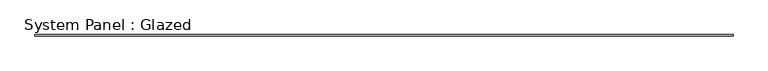
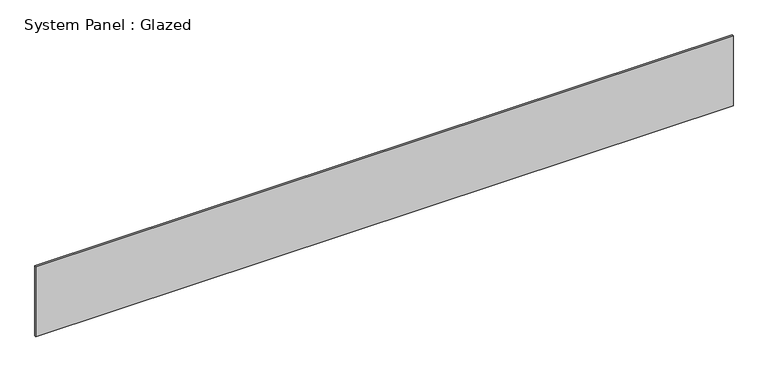
"""IFC4 building model written with IfcOpenShell, lengths in millimetres: plate geometry, System Panel : Glazed."""

from ifc_helpers import new_model, si_unit, origin, origin_with_axes, place, context, project, spatial, polyline, outline, extrude, source, transform, mapped, element, save


def system_panel_glazed_a411ffd8(model_context):
    return source(origin(), model_context, "Body", "SweptSolid", [
        extrude(outline(polyline([(6870.7, 19.05), (-6870.7, 19.05), (-6870.7, 44.45), (6870.7, 44.45), (6870.7, 19.05)])), origin_with_axes(), (0.0, 0.0, 1.0), 1460.5),
    ])


if __name__ == "__main__":
    model = new_model("IFC4")
    model_context = context("Model", 3, world=origin())
    ifc_project = project(units=[si_unit("LENGTHUNIT", "METRE", prefix="MILLI")], contexts=[model_context])
    site = spatial("IfcSite", under=ifc_project)
    building = spatial("IfcBuilding", under=site)
    placement = place(None, origin())
    system_panel_glazed_shape = system_panel_glazed_a411ffd8(model_context)
    element("IfcPlate", 1, ObjectType="System Panel : Glazed", at=placement, inside=building, context=model_context, shape_type="MappedRepresentation", body=[
        mapped(system_panel_glazed_shape, transform((0.0, 0.0, 0.0), x_axis=(1.0, 0.0, 0.0), y_axis=(0.0, 1.0, 0.0), z_axis=(0.0, 0.0, 1.0))),
    ])
    save(model, "model.ifc")

# Revit data of these elements
# Type "System Panel : Glazed"
#   Construction Type Id = "GSP4R"
#   Analytic Construction = "1/8 in Pilkington single glazing"
#   Visual Light Transmittance = 0.9
#   Solar Heat Gain Coefficient = 0.86
#   Heat Transfer Coefficient (U) = 1.18115 BTU/(h·ft²·°F)
# Element 1 (IfcPlate, "System Panel : Glazed")
#   Materials on its faces: "Glass"
# Materials
#   "Glass": class "Glass", colour RGB 0 128 192, transparency 0.75, Description = "Soda Lime Glass", Cost = 0
